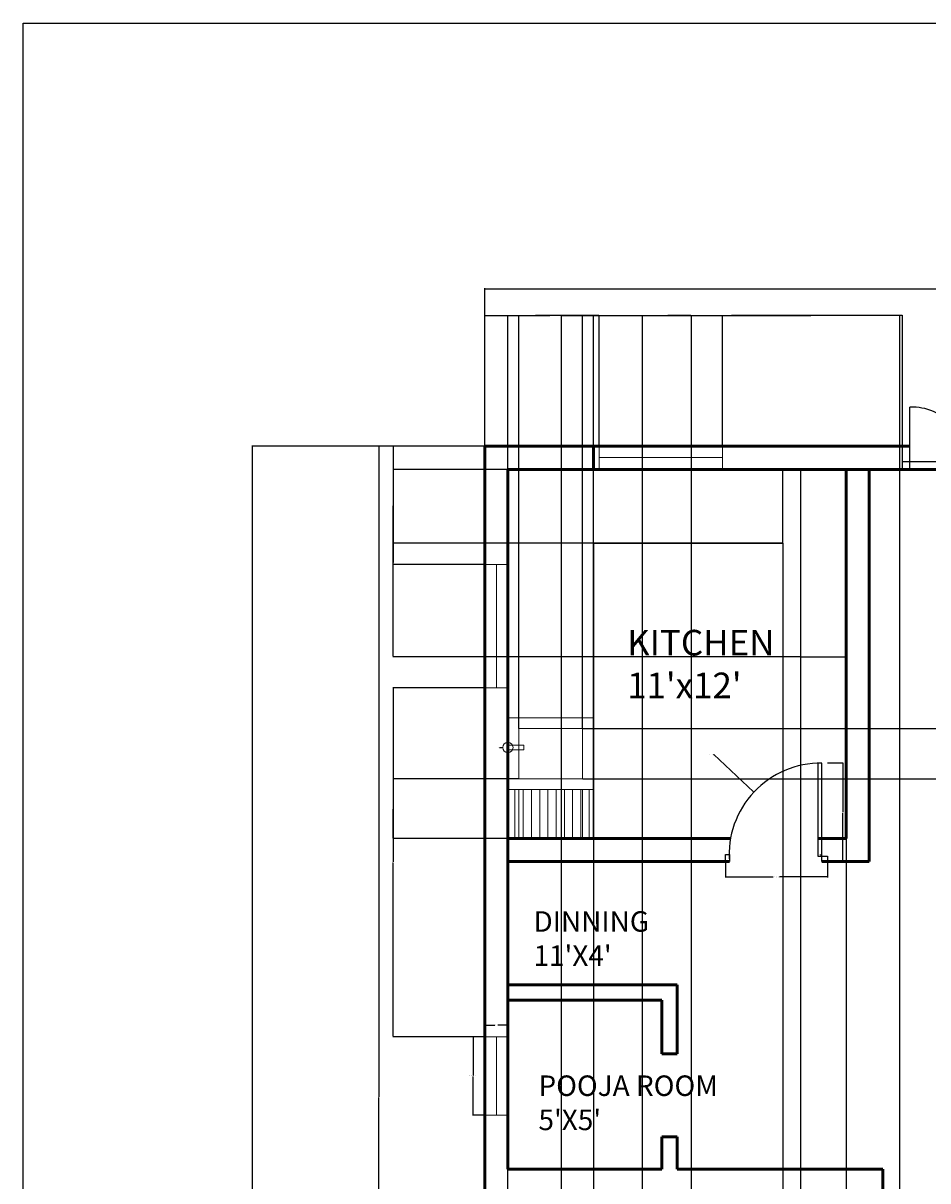
# Model space of a CAD drawing. Units: inches. Extents: x -177 to 2564, y -706 to 2548.
# Tile 3 of 4: x -177 to 176, y -266 to 186. Entities that reach past the tile are written whole.
import ezdxf

# ---------------------------------------------------------------- set-up
doc = ezdxf.new("R2010")
doc.units = ezdxf.units.IN
doc.header["$MEASUREMENT"] = 0
for name, color, linetype, lineweight in [('A-ANNO-DIMS', 2, 'Continuous', 18), ('A-ANNO-TTLB', 7, 'Continuous', 25), ('A-AREA-IDEN', 7, 'Continuous', 25), ('A-DOOR', 3, 'Continuous', 25), ('A-FLOR-CASE', 9, 'Continuous', 25), ('A-FLOR-FIXT', 8, 'Continuous', 18), ('A-GLAZ', 4, 'Continuous', 18), ('A-WALL', 7, 'Continuous', 50)]:
    doc.layers.add(name, color=color, linetype=linetype, lineweight=lineweight)
doc.styles.get("Standard").update_dxf_attribs({"font": 'arial.ttf'})
doc.dimstyles.get("Standard").update_dxf_attribs({"dimtxt": 0.18, "dimasz": 0.18, "dimexe": 0.18, "dimexo": 0.0625, "dimgap": 0.09, "dimtad": 0, "dimtih": 1, "dimtoh": 1, "dimdec": 0, "dimzin": 0, "dimdsep": 46, "dimlunit": 4, "dimtxsty": 'Standard', "dimcen": 0.09, "dimadec": 0, "dimazin": 0, "dimtfac": 1, "dimtdec": 0, "dimtofl": 0, "dimtmove": 0, "dimatfit": 3, "dimfxl": 1, "dimtolj": 1, "dimtzin": 0, "dimarcsym": 0})

# ---------------------------------------------------------------- blocks, each defined once
blk = doc.blocks.new('*D1')
at = {"layer": 'A-ANNO-DIMS', "color": 0, "lineweight": -2, "transparency": 16777216}
for p, q in [((3.47, 20.6), (3.47, 82.15)), ((3.65, 81.97), (192.07, 81.97)), ((381.29, 81.97), (192.87, 81.97)), ((381.47, 20.6), (381.47, 82.15))]:
    blk.add_line(p, q, dxfattribs=at)
at = {"layer": 'A-ANNO-DIMS', "color": 0, "transparency": 16777216}
for points in [[(3.65, 82), (3.65, 81.94), (3.47, 81.97)], [(381.29, 82), (381.29, 81.94), (381.47, 81.97)]]:
    blk.add_solid(points, dxfattribs=at)
at = {"layer": 'Defpoints', "color": 0, "transparency": 16777216}
for p in [(381.47, 81.97), (3.47, 20.54), (381.47, 20.54)]:
    blk.add_point(p, dxfattribs=at)
at = {"layer": 'A-ANNO-DIMS', "color": 0, "transparency": 16777216, "insert": (192.47, 81.97), "char_height": 0.18, "attachment_point": 5}
blk.add_mtext('\\A1;31\'-6"', dxfattribs=at)
blk = doc.blocks.new('*D2')
at = {"layer": 'A-ANNO-DIMS', "color": 0, "lineweight": -2, "transparency": 16777216}
for p, q in [((3.41, 20.54), (-38, 20.54)), ((-37.82, 20.36), (-37.82, -233.15)), ((-37.82, -487.01), (-37.82, -233.51)), ((3.41, -487.19), (-38, -487.19))]:
    blk.add_line(p, q, dxfattribs=at)
at = {"layer": 'A-ANNO-DIMS', "color": 0, "transparency": 16777216}
for points in [[(-37.85, 20.36), (-37.79, 20.36), (-37.82, 20.54)], [(-37.85, -487.01), (-37.79, -487.01), (-37.82, -487.19)]]:
    blk.add_solid(points, dxfattribs=at)
at = {"layer": 'Defpoints', "color": 0, "transparency": 16777216}
for p in [(3.47, 20.54), (-37.82, -487.19), (3.47, -487.19)]:
    blk.add_point(p, dxfattribs=at)
at = {"layer": 'A-ANNO-DIMS', "color": 0, "transparency": 16777216, "insert": (-37.82, -233.33), "char_height": 0.18, "attachment_point": 5}
blk.add_mtext('\\A1;42\'-4"', dxfattribs=at)
blk = doc.blocks.new('*D3')
at = {"layer": 'A-ANNO-DIMS', "color": 0, "lineweight": -2, "transparency": 16777216}
for p, q in [((3.41, 20.54), (-87.46, 20.54)), ((-87.28, 20.36), (-87.28, -294.78)), ((-87.28, -610.28), (-87.28, -295.15)), ((3.41, -610.46), (-87.46, -610.46))]:
    blk.add_line(p, q, dxfattribs=at)
at = {"layer": 'A-ANNO-DIMS', "color": 0, "transparency": 16777216}
for points in [[(-87.31, 20.36), (-87.25, 20.36), (-87.28, 20.54)], [(-87.31, -610.28), (-87.25, -610.28), (-87.28, -610.46)]]:
    blk.add_solid(points, dxfattribs=at)
at = {"layer": 'Defpoints', "color": 0, "transparency": 16777216}
for p in [(3.47, 20.54), (-87.28, -610.46), (3.47, -610.46)]:
    blk.add_point(p, dxfattribs=at)
at = {"layer": 'A-ANNO-DIMS', "color": 0, "transparency": 16777216, "insert": (-87.28, -294.96), "char_height": 0.18, "attachment_point": 5}
blk.add_mtext('\\A1;52\'-7"', dxfattribs=at)
blk = doc.blocks.new('WIN-48')
for p, q in [((0, 0), (9, 0)), ((9, 0), (4.59, 0)), ((4.59, 0), (4.59, -48.06)), ((9, -48.06), (0, -48.06))]:
    blk.add_line(p, q)
blk = doc.blocks.new('WIN-30')
for p, q in [((0, 30.54), (-9, 30.54)), ((-4.41, 0), (-4.41, 30.54)), ((0, 0), (-9, 0)), ((0, 0), (-4.41, 0))]:
    blk.add_line(p, q)
blk = doc.blocks.new('DOOR-SINGLE-36')
for p, q in [((1.57, 36.24), (0, 36.24)), ((0, 36.24), (0, 0)), ((1.57, -2.14), (1.57, 36.24)), ((1.57, 36.24), (1.57, 36.24)), ((-36.05, -2.14), (-36.05, 0.59)), ((-36.05, 0.59), (-34.54, 0.59)), ((-34.54, 0.59), (-34.54, -2.14)), ((0, 0), (3.72, 0)), ((3.72, 0), (3.72, -2.14)), ((3.72, -2.14), (1.57, -2.14))]:
    blk.add_line(p, q)
blk.add_arc((1.05, 0.56), 35.69, 89.1597, 184.3396)
blk = doc.blocks.new('DOOR-PAIR-44')
for p, q in [((0, 0), (0, 24.32)), ((44.01, 0), (44.01, 23.95)), ((-2.88, 0), (-2.88, 3.11)), ((-2.88, 3.11), (46.72, 3.11)), ((46.72, 0), (-2.88, 0)), ((-2.88, 0), (0, 0)), ((0, 0), (44.01, 0)), ((23.01, 0), (23.01, 3.55)), ((44.01, 0), (23.01, 0)), ((46.72, 0), (44.01, 0))]:
    blk.add_line(p, q)
for centre, radius, start, end in [((0.52, 1.77), 22.55, 355.4915, 91.326), ((45.7, 1.28), 22.73, 94.2755, 183.2347)]:
    blk.add_arc(centre, radius, start, end)
blk = doc.blocks.new('*D12')
at = {"layer": 'A-ANNO-DIMS', "color": 0, "lineweight": -2, "transparency": 16777216}
for p, q in [((3.41, -209.76), (-1.29, -209.76)), ((-1.11, -209.94), (-1.11, -224.85)), ((-1.11, -240.12), (-1.11, -225.22)), ((3.41, -240.3), (-1.29, -240.3))]:
    blk.add_line(p, q, dxfattribs=at)
at = {"layer": 'A-ANNO-DIMS', "color": 0, "transparency": 16777216}
for points in [[(-1.14, -209.94), (-1.08, -209.94), (-1.11, -209.76)], [(-1.14, -240.12), (-1.08, -240.12), (-1.11, -240.3)]]:
    blk.add_solid(points, dxfattribs=at)
at = {"layer": 'Defpoints', "color": 0, "transparency": 16777216}
for p in [(-1.11, -209.76), (3.47, -209.76), (3.47, -240.3)]:
    blk.add_point(p, dxfattribs=at)
at = {"layer": 'A-ANNO-DIMS', "color": 0, "transparency": 16777216, "insert": (-1.11, -225.03), "char_height": 0.18, "attachment_point": 5}
blk.add_mtext('\\A1;WINDOW W2 2\'-6 1/2" TYP.', dxfattribs=at)
blk = doc.blocks.new('*D13')
at = {"layer": 'A-ANNO-DIMS', "color": 0, "lineweight": -2, "transparency": 16777216}
for p, q in [((3.47, -209.7), (3.47, -205)), ((3.65, -205.18), (7.33, -205.18)), ((12.29, -205.18), (8.61, -205.18)), ((12.47, -209.7), (12.47, -205))]:
    blk.add_line(p, q, dxfattribs=at)
at = {"layer": 'A-ANNO-DIMS', "color": 0, "transparency": 16777216}
for points in [[(3.65, -205.15), (3.65, -205.21), (3.47, -205.18)], [(12.29, -205.15), (12.29, -205.21), (12.47, -205.18)]]:
    blk.add_solid(points, dxfattribs=at)
at = {"layer": 'Defpoints', "color": 0, "transparency": 16777216}
for p in [(12.47, -205.18), (3.47, -209.76), (12.47, -209.76)]:
    blk.add_point(p, dxfattribs=at)
at = {"layer": 'A-ANNO-DIMS', "color": 0, "transparency": 16777216, "insert": (7.97, -205.18), "char_height": 0.18, "attachment_point": 5}
blk.add_mtext('\\A1;0\'-9" TYP.', dxfattribs=at)
blk = doc.blocks.new('*D16')
at = {"layer": 'A-ANNO-DIMS', "color": 0, "lineweight": -2, "transparency": 16777216}
for p, q in [((97.36, -141.53), (97.36, -147.61)), ((137.13, -141.53), (137.13, -147.61)), ((97.54, -147.43), (116, -147.43)), ((136.95, -147.43), (118.49, -147.43))]:
    blk.add_line(p, q, dxfattribs=at)
at = {"layer": 'A-ANNO-DIMS', "color": 0, "transparency": 16777216}
for points in [[(97.54, -147.4), (97.54, -147.46), (97.36, -147.43)], [(136.95, -147.4), (136.95, -147.46), (137.13, -147.43)]]:
    blk.add_solid(points, dxfattribs=at)
at = {"layer": 'Defpoints', "color": 0, "transparency": 16777216}
for p in [(97.36, -141.46), (137.13, -141.46), (137.13, -147.43)]:
    blk.add_point(p, dxfattribs=at)
at = {"layer": 'A-ANNO-DIMS', "color": 0, "transparency": 16777216, "insert": (117.24, -147.43), "char_height": 0.18, "attachment_point": 5}
blk.add_mtext('\\A1;DOOR D1 3\'-4" TYP.', dxfattribs=at)
blk = doc.blocks.new('*D17')
at = {"layer": 'A-ANNO-DIMS', "color": 0, "lineweight": -2, "transparency": 16777216}
for p, q in [((137.19, -102.94), (143.28, -102.94)), ((143.1, -103.12), (143.1, -122.02)), ((143.1, -141.28), (143.1, -122.38)), ((137.19, -141.46), (143.28, -141.46))]:
    blk.add_line(p, q, dxfattribs=at)
at = {"layer": 'A-ANNO-DIMS', "color": 0, "transparency": 16777216}
for points in [[(143.07, -103.12), (143.13, -103.12), (143.1, -102.94)], [(143.07, -141.28), (143.13, -141.28), (143.1, -141.46)]]:
    blk.add_solid(points, dxfattribs=at)
at = {"layer": 'Defpoints', "color": 0, "transparency": 16777216}
for p in [(137.13, -102.94), (143.1, -102.94), (137.13, -141.46)]:
    blk.add_point(p, dxfattribs=at)
at = {"layer": 'A-ANNO-DIMS', "color": 0, "transparency": 16777216, "insert": (143.1, -122.2), "char_height": 0.18, "attachment_point": 5}
blk.add_mtext('\\A1;3\'-2 1/2" TYP.', dxfattribs=at)
blk = doc.blocks.new('*D22')
at = {"layer": 'A-ANNO-DIMS', "color": 0, "lineweight": -2, "transparency": 16777216}
for p, q in [((33.37, -291.35), (33.37, 71.74)), ((33.55, 71.56), (98.96, 71.56)), ((165.15, 71.56), (99.74, 71.56)), ((165.33, -291.35), (165.33, 71.74))]:
    blk.add_line(p, q, dxfattribs=at)
at = {"layer": 'A-ANNO-DIMS', "color": 0, "transparency": 16777216}
for points in [[(33.55, 71.59), (33.55, 71.53), (33.37, 71.56)], [(165.15, 71.59), (165.15, 71.53), (165.33, 71.56)]]:
    blk.add_solid(points, dxfattribs=at)
at = {"layer": 'Defpoints', "color": 0, "transparency": 16777216}
for p in [(165.33, 71.56), (33.37, -291.42), (165.33, -291.42)]:
    blk.add_point(p, dxfattribs=at)
at = {"layer": 'A-ANNO-DIMS', "color": 0, "transparency": 16777216, "insert": (99.35, 71.56), "char_height": 0.18, "attachment_point": 5}
blk.add_mtext('\\A1;11\'-0"', dxfattribs=at)
blk = doc.blocks.new('*D26')
at = {"layer": 'A-ANNO-DIMS', "color": 0, "lineweight": -2, "transparency": 16777216}
for p, q in [((64.94, -324.62), (64.94, 71.74)), ((65.12, 71.56), (74.18, 71.56)), ((83.88, 71.56), (74.82, 71.56)), ((84.06, -343.44), (84.06, 71.74))]:
    blk.add_line(p, q, dxfattribs=at)
at = {"layer": 'A-ANNO-DIMS', "color": 0, "transparency": 16777216}
for points in [[(65.12, 71.59), (65.12, 71.53), (64.94, 71.56)], [(83.88, 71.59), (83.88, 71.53), (84.06, 71.56)]]:
    blk.add_solid(points, dxfattribs=at)
at = {"layer": 'Defpoints', "color": 0, "transparency": 16777216}
for p in [(84.06, 71.56), (64.94, -324.69), (84.06, -343.5)]:
    blk.add_point(p, dxfattribs=at)
at = {"layer": 'A-ANNO-DIMS', "color": 0, "transparency": 16777216, "insert": (74.5, 71.56), "char_height": 0.18, "attachment_point": 5}
blk.add_mtext('\\A1;1\'-7"', dxfattribs=at)
blk = doc.blocks.new('*D28')
at = {"layer": 'A-ANNO-DIMS', "color": 0, "lineweight": -2, "transparency": 16777216}
for p, q in [((12.47, -270.4), (12.47, 71.74)), ((12.65, 71.56), (22.6, 71.56)), ((33.19, 71.56), (23.24, 71.56)), ((33.37, -291.35), (33.37, 71.74))]:
    blk.add_line(p, q, dxfattribs=at)
at = {"layer": 'A-ANNO-DIMS', "color": 0, "transparency": 16777216}
for points in [[(12.65, 71.59), (12.65, 71.53), (12.47, 71.56)], [(33.19, 71.59), (33.19, 71.53), (33.37, 71.56)]]:
    blk.add_solid(points, dxfattribs=at)
at = {"layer": 'Defpoints', "color": 0, "transparency": 16777216}
for p in [(33.37, 71.56), (12.47, -270.46), (33.37, -291.42)]:
    blk.add_point(p, dxfattribs=at)
at = {"layer": 'A-ANNO-DIMS', "color": 0, "transparency": 16777216, "insert": (22.92, 71.56), "char_height": 0.18, "attachment_point": 5}
blk.add_mtext('\\A1;1\'-9"', dxfattribs=at)
blk = doc.blocks.new('*D30')
at = {"layer": 'A-ANNO-DIMS', "color": 0, "lineweight": -2, "transparency": 16777216}
for p, q in [((12.47, -85.26), (12.47, 71.74)), ((12.65, 71.56), (28.65, 71.56)), ((45.73, 71.56), (29.73, 71.56)), ((45.91, -85.26), (45.91, 71.74))]:
    blk.add_line(p, q, dxfattribs=at)
at = {"layer": 'A-ANNO-DIMS', "color": 0, "transparency": 16777216}
for points in [[(12.65, 71.59), (12.65, 71.53), (12.47, 71.56)], [(45.73, 71.59), (45.73, 71.53), (45.91, 71.56)]]:
    blk.add_solid(points, dxfattribs=at)
at = {"layer": 'Defpoints', "color": 0, "transparency": 16777216}
for p in [(45.91, 71.56), (12.47, -85.33), (45.91, -85.33)]:
    blk.add_point(p, dxfattribs=at)
at = {"layer": 'A-ANNO-DIMS', "color": 0, "transparency": 16777216, "insert": (29.19, 71.56), "char_height": 0.18, "attachment_point": 5}
blk.add_mtext('\\A1;2\'-9 1/2"', dxfattribs=at)
blk = doc.blocks.new('*D31')
at = {"layer": 'A-ANNO-DIMS', "color": 0, "lineweight": -2, "transparency": 16777216}
for p, q in [((119.69, 11.54), (-32.41, 11.54)), ((-32.23, 11.36), (-32.23, -2.66)), ((-32.23, -17.03), (-32.23, -3.02)), ((119.69, -17.21), (-32.41, -17.21))]:
    blk.add_line(p, q, dxfattribs=at)
at = {"layer": 'A-ANNO-DIMS', "color": 0, "transparency": 16777216}
for points in [[(-32.26, 11.36), (-32.2, 11.36), (-32.23, 11.54)], [(-32.26, -17.03), (-32.2, -17.03), (-32.23, -17.21)]]:
    blk.add_solid(points, dxfattribs=at)
at = {"layer": 'Defpoints', "color": 0, "transparency": 16777216}
for p in [(119.76, 11.54), (-32.23, -17.21), (119.76, -17.21)]:
    blk.add_point(p, dxfattribs=at)
at = {"layer": 'A-ANNO-DIMS', "color": 0, "transparency": 16777216, "insert": (-32.23, -2.84), "char_height": 0.18, "attachment_point": 5}
blk.add_mtext('\\A1;2\'-4 1/2"', dxfattribs=at)
blk = doc.blocks.new('*D32')
at = {"layer": 'A-ANNO-DIMS', "color": 0, "lineweight": -2, "transparency": 16777216}
for p, q in [((45.91, -17.28), (45.91, -646.34)), ((119.76, -17.28), (119.76, -646.34)), ((46.09, -646.16), (82.5, -646.16)), ((119.58, -646.16), (83.16, -646.16))]:
    blk.add_line(p, q, dxfattribs=at)
at = {"layer": 'A-ANNO-DIMS', "color": 0, "transparency": 16777216}
for points in [[(46.09, -646.13), (46.09, -646.19), (45.91, -646.16)], [(119.58, -646.13), (119.58, -646.19), (119.76, -646.16)]]:
    blk.add_solid(points, dxfattribs=at)
at = {"layer": 'Defpoints', "color": 0, "transparency": 16777216}
for p in [(45.91, -17.21), (119.76, -17.21), (119.76, -646.16)]:
    blk.add_point(p, dxfattribs=at)
at = {"layer": 'A-ANNO-DIMS', "color": 0, "transparency": 16777216, "insert": (82.83, -646.16), "char_height": 0.18, "attachment_point": 5}
blk.add_mtext('\\A1;6\'-2"', dxfattribs=at)
blk = doc.blocks.new('*D33')
at = {"layer": 'A-ANNO-DIMS', "color": 0, "lineweight": -2, "transparency": 16777216}
for p, q in [((126.64, -61.62), (126.64, -646.34)), ((144.47, -61.62), (144.47, -646.34)), ((126.82, -646.16), (135.24, -646.16)), ((144.29, -646.16), (135.88, -646.16))]:
    blk.add_line(p, q, dxfattribs=at)
at = {"layer": 'A-ANNO-DIMS', "color": 0, "transparency": 16777216}
for points in [[(126.82, -646.13), (126.82, -646.19), (126.64, -646.16)], [(144.29, -646.13), (144.29, -646.19), (144.47, -646.16)]]:
    blk.add_solid(points, dxfattribs=at)
at = {"layer": 'Defpoints', "color": 0, "transparency": 16777216}
for p in [(126.64, -61.56), (144.47, -61.56), (144.47, -646.16)]:
    blk.add_point(p, dxfattribs=at)
at = {"layer": 'A-ANNO-DIMS', "color": 0, "transparency": 16777216, "insert": (135.56, -646.16), "char_height": 0.18, "attachment_point": 5}
blk.add_mtext('\\A1;1\'-6"', dxfattribs=at)
blk = doc.blocks.new('*D34')
at = {"layer": 'A-ANNO-DIMS', "color": 0, "lineweight": -2, "transparency": 16777216}
for p, q in [((126.58, 11.54), (-32.41, 11.54)), ((-32.23, 11.36), (-32.23, -24.83)), ((-32.23, -61.38), (-32.23, -25.19)), ((126.58, -61.56), (-32.41, -61.56))]:
    blk.add_line(p, q, dxfattribs=at)
at = {"layer": 'A-ANNO-DIMS', "color": 0, "transparency": 16777216}
for points in [[(-32.26, 11.36), (-32.2, 11.36), (-32.23, 11.54)], [(-32.26, -61.38), (-32.2, -61.38), (-32.23, -61.56)]]:
    blk.add_solid(points, dxfattribs=at)
at = {"layer": 'Defpoints', "color": 0, "transparency": 16777216}
for p in [(-32.23, 11.54), (126.64, 11.54), (126.64, -61.56)]:
    blk.add_point(p, dxfattribs=at)
at = {"layer": 'A-ANNO-DIMS', "color": 0, "transparency": 16777216, "insert": (-32.23, -25.01), "char_height": 0.18, "attachment_point": 5}
blk.add_mtext('\\A1;6\'-1"', dxfattribs=at)
blk = doc.blocks.new('*D35')
at = {"layer": 'A-ANNO-DIMS', "color": 0, "lineweight": -2, "transparency": 16777216}
for p, q in [((16.73, -89.52), (16.73, 71.74)), ((16.91, 71.56), (28.86, 71.56)), ((41.47, 71.56), (29.52, 71.56)), ((41.65, -89.52), (41.65, 71.74))]:
    blk.add_line(p, q, dxfattribs=at)
at = {"layer": 'A-ANNO-DIMS', "color": 0, "transparency": 16777216}
for points in [[(16.91, 71.59), (16.91, 71.53), (16.73, 71.56)], [(41.47, 71.59), (41.47, 71.53), (41.65, 71.56)]]:
    blk.add_solid(points, dxfattribs=at)
at = {"layer": 'Defpoints', "color": 0, "transparency": 16777216}
for p in [(41.65, 71.56), (16.73, -89.59), (41.65, -89.59)]:
    blk.add_point(p, dxfattribs=at)
at = {"layer": 'A-ANNO-DIMS', "color": 0, "transparency": 16777216, "insert": (29.19, 71.56), "char_height": 0.18, "attachment_point": 5}
blk.add_mtext('\\A1;2\'-1"', dxfattribs=at)
blk = doc.blocks.new('*D36')
at = {"layer": 'A-ANNO-DIMS', "color": 0, "lineweight": -2, "transparency": 16777216}
for p, q in [((41.71, -89.59), (417.35, -89.59)), ((417.17, -89.77), (417.17, -99.17)), ((417.17, -108.95), (417.17, -99.54)), ((41.71, -109.13), (417.35, -109.13))]:
    blk.add_line(p, q, dxfattribs=at)
at = {"layer": 'A-ANNO-DIMS', "color": 0, "transparency": 16777216}
for points in [[(417.14, -89.77), (417.2, -89.77), (417.17, -89.59)], [(417.14, -108.95), (417.2, -108.95), (417.17, -109.13)]]:
    blk.add_solid(points, dxfattribs=at)
at = {"layer": 'Defpoints', "color": 0, "transparency": 16777216}
for p in [(41.65, -89.59), (41.65, -109.13), (417.17, -109.13)]:
    blk.add_point(p, dxfattribs=at)
at = {"layer": 'A-ANNO-DIMS', "color": 0, "transparency": 16777216, "insert": (417.17, -99.36), "char_height": 0.18, "attachment_point": 5}
blk.add_mtext('\\A1;1\'-7 1/2"', dxfattribs=at)
blk = doc.blocks.new('*D37')
at = {"layer": 'A-ANNO-DIMS', "color": 0, "lineweight": -2, "transparency": 16777216}
for p, q in [((16.67, -109.13), (-32.41, -109.13)), ((-32.23, -109.31), (-32.23, -120.61)), ((-32.23, -132.28), (-32.23, -120.98)), ((12.41, -132.46), (-32.41, -132.46))]:
    blk.add_line(p, q, dxfattribs=at)
at = {"layer": 'A-ANNO-DIMS', "color": 0, "transparency": 16777216}
for points in [[(-32.26, -109.31), (-32.2, -109.31), (-32.23, -109.13)], [(-32.26, -132.28), (-32.2, -132.28), (-32.23, -132.46)]]:
    blk.add_solid(points, dxfattribs=at)
at = {"layer": 'Defpoints', "color": 0, "transparency": 16777216}
for p in [(-32.23, -109.13), (16.73, -109.13), (12.47, -132.46)]:
    blk.add_point(p, dxfattribs=at)
at = {"layer": 'A-ANNO-DIMS', "color": 0, "transparency": 16777216, "insert": (-32.23, -120.8), "char_height": 0.18, "attachment_point": 5}
blk.add_mtext('\\A1;1\'-11 1/2"', dxfattribs=at)
blk = doc.blocks.new('*D50')
at = {"layer": 'A-ANNO-DIMS', "color": 0, "lineweight": -2, "transparency": 16777216}
for p, q in [((3.47, 20.6), (3.47, 71.74)), ((3.65, 71.56), (25.24, 71.56)), ((47.91, 71.56), (26.32, 71.56)), ((48.09, 20.6), (48.09, 71.74))]:
    blk.add_line(p, q, dxfattribs=at)
at = {"layer": 'A-ANNO-DIMS', "color": 0, "transparency": 16777216}
for points in [[(3.65, 71.59), (3.65, 71.53), (3.47, 71.56)], [(47.91, 71.59), (47.91, 71.53), (48.09, 71.56)]]:
    blk.add_solid(points, dxfattribs=at)
at = {"layer": 'Defpoints', "color": 0, "transparency": 16777216}
for p in [(48.09, 71.56), (3.47, 20.54), (48.09, 20.54)]:
    blk.add_point(p, dxfattribs=at)
at = {"layer": 'A-ANNO-DIMS', "color": 0, "transparency": 16777216, "insert": (25.78, 71.56), "char_height": 0.18, "attachment_point": 5}
blk.add_mtext('\\A1;3\'-8 1/2"', dxfattribs=at)
blk = doc.blocks.new('*D51')
at = {"layer": 'A-ANNO-DIMS', "color": 0, "lineweight": -2, "transparency": 16777216}
for p, q in [((96.15, 20.6), (96.15, 71.74)), ((96.33, 71.56), (130.67, 71.56)), ((166.23, 71.56), (131.89, 71.56)), ((166.41, 20.6), (166.41, 71.74))]:
    blk.add_line(p, q, dxfattribs=at)
at = {"layer": 'A-ANNO-DIMS', "color": 0, "transparency": 16777216}
for points in [[(96.33, 71.59), (96.33, 71.53), (96.15, 71.56)], [(166.23, 71.59), (166.23, 71.53), (166.41, 71.56)]]:
    blk.add_solid(points, dxfattribs=at)
at = {"layer": 'Defpoints', "color": 0, "transparency": 16777216}
for p in [(166.41, 71.56), (96.15, 20.54), (166.41, 20.54)]:
    blk.add_point(p, dxfattribs=at)
at = {"layer": 'A-ANNO-DIMS', "color": 0, "transparency": 16777216, "insert": (131.28, 71.56), "char_height": 0.18, "attachment_point": 5}
blk.add_mtext('\\A1;5\'-10 1/2"', dxfattribs=at)
blk = doc.blocks.new('*D53')
at = {"layer": 'A-ANNO-DIMS', "color": 0, "lineweight": -2, "transparency": 16777216}
for p, q in [((3.41, 20.54), (-32.41, 20.54)), ((-32.23, 20.36), (-32.23, -2.36)), ((-32.23, -25.45), (-32.23, -2.73)), ((3.41, -25.63), (-32.41, -25.63))]:
    blk.add_line(p, q, dxfattribs=at)
at = {"layer": 'A-ANNO-DIMS', "color": 0, "transparency": 16777216}
for points in [[(-32.26, 20.36), (-32.2, 20.36), (-32.23, 20.54)], [(-32.26, -25.45), (-32.2, -25.45), (-32.23, -25.63)]]:
    blk.add_solid(points, dxfattribs=at)
at = {"layer": 'Defpoints', "color": 0, "transparency": 16777216}
for p in [(-32.23, 20.54), (3.47, 20.54), (3.47, -25.63)]:
    blk.add_point(p, dxfattribs=at)
at = {"layer": 'A-ANNO-DIMS', "color": 0, "transparency": 16777216, "insert": (-32.23, -2.55), "char_height": 0.18, "attachment_point": 5}
blk.add_mtext('\\A1;3\'-10"', dxfattribs=at)
blk = doc.blocks.new('*D55')
at = {"layer": 'A-ANNO-DIMS', "color": 0, "lineweight": -2, "transparency": 16777216}
for p, q in [((3.41, -73.69), (-32.41, -73.69)), ((-32.23, -73.87), (-32.23, -141.54)), ((-32.23, -209.58), (-32.23, -141.9)), ((3.41, -209.76), (-32.41, -209.76))]:
    blk.add_line(p, q, dxfattribs=at)
at = {"layer": 'A-ANNO-DIMS', "color": 0, "transparency": 16777216}
for points in [[(-32.26, -73.87), (-32.2, -73.87), (-32.23, -73.69)], [(-32.26, -209.58), (-32.2, -209.58), (-32.23, -209.76)]]:
    blk.add_solid(points, dxfattribs=at)
at = {"layer": 'Defpoints', "color": 0, "transparency": 16777216}
for p in [(3.47, -73.69), (-32.23, -209.76), (3.47, -209.76)]:
    blk.add_point(p, dxfattribs=at)
at = {"layer": 'A-ANNO-DIMS', "color": 0, "transparency": 16777216, "insert": (-32.23, -141.72), "char_height": 0.18, "attachment_point": 5}
blk.add_mtext('\\A1;11\'-4"', dxfattribs=at)
blk = doc.blocks.new('*D62')
at = {"layer": 'A-ANNO-DIMS', "color": 0, "lineweight": -2, "transparency": 16777216}
for p, q in [((9.26, -96.93), (10.28, -96.94)), ((12.38, -96.96), (12.56, -96.96)), ((12.47, -97.05), (12.47, -96.87))]:
    blk.add_line(p, q, dxfattribs=at)
at = {"layer": 'A-ANNO-DIMS', "color": 0, "transparency": 16777216}
blk.add_solid([(10.28, -96.91), (10.28, -96.97), (10.46, -96.94)], dxfattribs=at)
at = {"layer": 'Defpoints', "color": 0, "transparency": 16777216}
for p in [(10.46, -96.94), (14.48, -96.98)]:
    blk.add_point(p, dxfattribs=at)
at = {"layer": 'A-ANNO-DIMS', "color": 0, "transparency": 16777216, "insert": (8.83, -96.93), "char_height": 0.18, "attachment_point": 5}
blk.add_mtext('\\A1;∅0\'-4"', dxfattribs=at)
blk = doc.blocks.new('*D63')
at = {"layer": 'A-ANNO-DIMS', "color": 0, "lineweight": -2, "transparency": 16777216}
for p, q in [((92.69, -99.64), (92.87, -99.64)), ((92.87, -99.64), (108.33, -114.19)), ((134.37, -138.76), (134.55, -138.76)), ((134.46, -138.85), (134.46, -138.67))]:
    blk.add_line(p, q, dxfattribs=at)
at = {"layer": 'A-ANNO-DIMS', "color": 0, "transparency": 16777216}
blk.add_solid([(108.36, -114.17), (108.31, -114.21), (108.47, -114.31)], dxfattribs=at)
at = {"layer": 'Defpoints', "color": 0, "transparency": 16777216}
for p in [(108.47, -114.31), (134.46, -138.76)]:
    blk.add_point(p, dxfattribs=at)
at = {"layer": 'A-ANNO-DIMS', "color": 0, "transparency": 16777216, "insert": (91.8, -99.64), "char_height": 0.18, "attachment_point": 5}
blk.add_mtext('\\A1;6X R2\'-11 1/2"', dxfattribs=at)

msp = doc.modelspace()

# ---------------------------------------------------------------- linework, layer by layer
at = {"layer": 'A-ANNO-TTLB'}
msp.add_lwpolyline([(-176.6, 185.58), (523.32, 185.58), (523.32, -705.52), (-176.6, -705.52)], close=True, dxfattribs=at)
at = {"layer": 'A-DOOR'}
for p, q in [((166.41, 11.54), (166.41, 20.54)), ((97.36, -141.46), (98.87, -141.46))]:
    msp.add_line(p, q, dxfattribs=at)
at = {"layer": 'A-FLOR-CASE'}
for p, q in [((119.76, -17.21), (119.76, 11.54)), ((119.76, 11.54), (126.64, 11.54)), ((126.64, 11.54), (126.64, -61.56)), ((45.91, -132.46), (45.91, -17.21)), ((45.91, -17.21), (119.76, -17.21)), ((126.64, -61.56), (144.47, -61.56)), ((12.47, -132.46), (45.91, -132.46))]:
    msp.add_line(p, q, dxfattribs=at)
msp.add_lwpolyline([(45.91, -17.21), (45.91, -132.46), (12.47, -132.46), (12.47, 11.54)], dxfattribs=at)
at = {"layer": 'A-FLOR-FIXT'}
for p, q in [((45.91, -85.33), (12.47, -85.33)), ((12.47, -85.33), (12.47, -98.97)), ((12.47, -85.33), (12.47, -96.02)), ((45.91, -132.46), (45.91, -85.33)), ((41.65, -89.59), (16.73, -89.59)), ((16.73, -89.59), (16.73, -109.13)), ((41.65, -109.13), (41.65, -89.59)), ((12.47, -96.02), (18.74, -96.02)), ((18.74, -97.91), (12.47, -97.91)), ((18.74, -96.02), (18.74, -97.91)), ((16.73, -109.13), (41.65, -109.13)), ((12.47, -132.46), (12.47, -113.39)), ((12.47, -113.39), (45.91, -113.39)), ((12.47, -113.39), (15.24, -113.39)), ((12.47, -113.39), (12.47, -132.46)), ((15.24, -113.39), (15.24, -132.46)), ((16.73, -113.39), (16.73, -132.46)), ((18.46, -113.39), (18.46, -132.46)), ((21.67, -113.39), (21.67, -132.46)), ((24.88, -113.39), (24.88, -132.46)), ((28.09, -113.39), (28.09, -132.46)), ((31.31, -113.39), (31.31, -132.46)), ((34.52, -113.39), (34.52, -132.46)), ((37.73, -113.39), (37.73, -132.46)), ((40.95, -113.39), (40.95, -132.46)), ((41.65, -132.46), (41.65, -113.39)), ((44.16, -113.39), (44.16, -132.46)), ((12.47, -132.46), (45.91, -132.46))]:
    msp.add_line(p, q, dxfattribs=at)
msp.add_circle((12.47, -96.96), 2.01, dxfattribs=at)
at = {"layer": 'A-GLAZ'}
for p, q in [((3.47, -73.69), (12.47, -73.69)), ((3.47, -209.76), (3.47, -240.3))]:
    msp.add_line(p, q, dxfattribs=at)
at = {"layer": 'A-WALL'}
for p, q in [((3.47, -483.46), (3.47, 20.54)), ((3.47, 20.54), (12.47, 20.54)), ((12.47, 20.54), (169.3, 20.54)), ((12.47, 11.54), (372.47, 11.54)), ((12.47, 11.54), (12.47, -261.46)), ((12.47, 11.54), (144.47, 11.54)), ((144.47, 11.54), (144.47, -132.46)), ((153.47, -141.46), (153.47, 11.54)), ((12.47, -132.46), (12.47, -141.46)), ((99.33, -132.46), (12.47, -132.46)), ((144.47, -132.46), (133.41, -132.46)), ((12.47, -141.46), (98.87, -141.46)), ((12.47, -141.46), (12.47, -189.46)), ((134.98, -141.46), (144.47, -141.46)), ((144.47, -141.46), (153.47, -141.46)), ((144.47, -141.46), (153.47, -141.46)), ((12.47, -189.46), (72.47, -189.46)), ((72.47, -189.46), (78.47, -189.46)), ((78.47, -189.46), (78.47, -216.41)), ((72.47, -195.46), (12.47, -195.46)), ((12.47, -195.46), (12.47, -255.46)), ((12.47, -195.46), (12.47, -209.76)), ((72.47, -216.41), (72.47, -195.46)), ((78.47, -216.41), (72.47, -216.41)), ((72.47, -255.46), (72.47, -248.84)), ((72.47, -248.84), (78.5, -248.84)), ((78.5, -248.84), (78.5, -261.46)), ((72.47, -255.46), (72.47, -261.46)), ((72.47, -261.46), (12.47, -261.46)), ((12.47, -261.46), (72.47, -261.46)), ((78.5, -261.46), (158.78, -261.46)), ((158.78, -261.46), (158.78, -270.46))]:
    msp.add_line(p, q, dxfattribs=at)
msp.add_lwpolyline([(12.47, 20.54), (45.91, 20.54), (45.91, 11.54)], dxfattribs=at)

# ---------------------------------------------------------------- block references
at = {"layer": 'A-DOOR'}
for name, p in [('DOOR-PAIR-44', (169.3, 11.54)), ('DOOR-SINGLE-36', (133.41, -139.32))]:
    msp.add_blockref(name, p, dxfattribs=at)
at = {"layer": 'A-GLAZ', "rotation": 89.99999999999987}
msp.add_blockref('WIN-48', (48.09, 11.54), dxfattribs=at)
at = {"layer": 'A-GLAZ'}
for name, p in [('WIN-48', (3.47, -25.63)), ('WIN-30', (12.47, -240.3))]:
    msp.add_blockref(name, p, dxfattribs=at)

# ---------------------------------------------------------------- texts
at = {"layer": 'A-AREA-IDEN', "attachment_point": 1}
for s, width, insert, char_height in [("KITCHEN \\P11'x12'", 38.4012, (58.98, -51.06), 10), ("DINNING\\P11'X4'", 0.2169, (22.47, -160.8), 8)]:
    msp.add_mtext_dynamic_manual_height_columns(s, width=width, gutter_width=1, heights=[0], dxfattribs=dict(at, insert=insert, char_height=char_height))
at = {"layer": 'A-AREA-IDEN', "insert": (24.41, -224.86), "char_height": 8, "attachment_point": 1}
msp.add_mtext("POOJA ROOM\\P5'X5'", dxfattribs=at)

# ---------------------------------------------------------------- dimensions: what is measured, and where the dimension line sits
at = {"layer": 'A-ANNO-DIMS'}
for base, p1, p2, override, picture, middle in [((381.47, 81.97), (3.47, 20.54), (381.47, 20.54), {"dimclrd": 0, "dimclre": 0, "dimclrt": 0}, '*D1', (192.47, 81.97)), ((48.09, 71.56), (3.47, 20.54), (48.09, 20.54), {"dimdec": 1, "dimlfac": 1, "dimrnd": 0, "dimzin": 1, "dimdsep": 46, "dimlunit": 4, "dimfrac": 2}, '*D50', (25.78, 71.56)), ((45.91, 71.56), (12.47, -85.33), (45.91, -85.33), {"dimdec": 1, "dimlfac": 1, "dimrnd": 0, "dimzin": 1, "dimdsep": 46, "dimlunit": 4, "dimfrac": 2}, '*D30', (29.19, 71.56)), ((33.37, 71.56), (12.47, -270.46), (33.37, -291.42), {"dimdec": 1, "dimlfac": 1, "dimrnd": 0, "dimzin": 1, "dimdsep": 46, "dimlunit": 4, "dimfrac": 2}, '*D28', (22.92, 71.56)), ((41.65, 71.56), (16.73, -89.59), (41.65, -89.59), {"dimdec": 1, "dimlfac": 1, "dimrnd": 0, "dimzin": 1, "dimdsep": 46, "dimlunit": 4, "dimfrac": 2}, '*D35', (29.19, 71.56)), ((165.33, 71.56), (33.37, -291.42), (165.33, -291.42), {"dimdec": 1, "dimlfac": 1, "dimrnd": 0, "dimzin": 1, "dimdsep": 46, "dimlunit": 4, "dimfrac": 2}, '*D22', (99.35, 71.56)), ((84.06, 71.56), (64.94, -324.69), (84.06, -343.5), {"dimdec": 1, "dimlfac": 1, "dimrnd": 0, "dimzin": 1, "dimdsep": 46, "dimlunit": 4, "dimfrac": 2}, '*D26', (74.5, 71.56)), ((166.41, 71.56), (96.15, 20.54), (166.41, 20.54), {"dimdec": 1, "dimlfac": 1, "dimrnd": 0, "dimzin": 1, "dimdsep": 46, "dimlunit": 4, "dimfrac": 2}, '*D51', (131.28, 71.56)), ((119.7563, -646.1645), (45.9113, -17.2143), (119.7563, -17.2143), {"dimdec": 1, "dimlfac": 1, "dimrnd": 0, "dimzin": 1, "dimdsep": 46, "dimlunit": 4, "dimfrac": 2}, '*D32', (82.8338, -646.1645)), ((144.47, -646.16), (126.64, -61.56), (144.47, -61.56), {"dimdec": 1, "dimlfac": 1, "dimrnd": 0, "dimzin": 1, "dimdsep": 46, "dimlunit": 4, "dimfrac": 2}, '*D33', (135.56, -646.16))]:
    dim = msp.add_linear_dim(base=base, p1=p1, p2=p2, dimstyle='Standard', override=override, dxfattribs=at)
    dim.commit()
    dim.dimension.update_dxf_attribs({"geometry": picture, "text_midpoint": middle})
for base, p1, p2, override, picture, middle in [((-87.28, -610.46), (3.47, 20.54), (3.47, -610.46), {"dimclrd": 0, "dimclre": 0, "dimclrt": 0}, '*D3', (-87.28, -294.96)), ((-37.82, -487.19), (3.47, 20.54), (3.47, -487.19), {"dimclrd": 0, "dimclre": 0, "dimclrt": 0}, '*D2', (-37.82, -233.33)), ((-32.23, 20.54), (3.47, -25.63), (3.47, 20.54), {"dimdec": 1, "dimlfac": 1, "dimrnd": 0, "dimzin": 1, "dimdsep": 46, "dimlunit": 4, "dimfrac": 2}, '*D53', (-32.23, -2.55)), ((-32.2267, -17.2143), (119.7563, 11.5355), (119.7563, -17.2143), {"dimdec": 1, "dimlfac": 1, "dimrnd": 0, "dimzin": 1, "dimdsep": 46, "dimlunit": 4, "dimfrac": 2}, '*D31', (-32.2267, -2.8394)), ((-32.23, 11.54), (126.64, -61.56), (126.64, 11.54), {"dimdec": 1, "dimlfac": 1, "dimrnd": 0, "dimzin": 1, "dimdsep": 46, "dimlunit": 4, "dimfrac": 2}, '*D34', (-32.23, -25.01)), ((-32.23, -209.76), (3.47, -73.69), (3.47, -209.76), {"dimdec": 1, "dimlfac": 1, "dimrnd": 0, "dimzin": 1, "dimdsep": 46, "dimlunit": 4, "dimfrac": 2}, '*D55', (-32.23, -141.72)), ((417.17, -109.13), (41.65, -89.59), (41.65, -109.13), {"dimdec": 1, "dimlfac": 1, "dimrnd": 0, "dimzin": 1, "dimdsep": 46, "dimlunit": 4, "dimfrac": 2}, '*D36', (417.17, -99.36)), ((-32.23, -109.13), (12.47, -132.46), (16.73, -109.13), {"dimdec": 1, "dimlfac": 1, "dimrnd": 0, "dimzin": 1, "dimdsep": 46, "dimlunit": 4, "dimfrac": 2}, '*D37', (-32.23, -120.8))]:
    dim = msp.add_linear_dim(base=base, p1=p1, p2=p2, angle=90, dimstyle='Standard', override=override, dxfattribs=at)
    dim.commit()
    dim.dimension.update_dxf_attribs({"geometry": picture, "text_midpoint": middle})
dim = msp.add_diameter_dim_2p(p1=(14.48, -96.98), p2=(10.46, -96.94), dimstyle='Standard', override={"dimdec": 1, "dimlfac": 1, "dimrnd": 0, "dimzin": 1, "dimdsep": 46, "dimlunit": 4, "dimfrac": 2}, dxfattribs=at)
dim.commit()
dim.dimension.update_dxf_attribs({"geometry": '*D62', "text_midpoint": (9.26, -96.93), "dimtype": 163})
dim = msp.add_radius_dim(center=(134.46, -138.76), mpoint=(108.47, -114.31), text='6X <>', dimstyle='Standard', override={"dimdec": 1, "dimlfac": 1, "dimrnd": 0, "dimzin": 1, "dimdsep": 46, "dimlunit": 4, "dimfrac": 2}, dxfattribs=at)
dim.commit()
dim.dimension.update_dxf_attribs({"geometry": '*D63', "text_midpoint": (91.8, -99.64), "dimtype": 164})
for base, p1, p2, text, picture, middle in [((143.1, -102.94), (137.13, -141.46), (137.13, -102.94), '<> TYP.', '*D17', (143.1, -122.2)), ((-1.11, -209.76), (3.47, -240.3), (3.47, -209.76), 'WINDOW W2 <> TYP.', '*D12', (-1.11, -225.03))]:
    dim = msp.add_linear_dim(base=base, p1=p1, p2=p2, angle=90, text=text, dimstyle='Standard', override={"dimdec": 1, "dimlfac": 1, "dimrnd": 0, "dimzin": 1, "dimdsep": 46, "dimlunit": 4, "dimfrac": 2}, dxfattribs=at)
    dim.commit()
    dim.dimension.update_dxf_attribs({"geometry": picture, "text_midpoint": middle})
for base, p1, p2, text, picture, middle in [((137.13, -147.43), (97.36, -141.46), (137.13, -141.46), 'DOOR D1 <> TYP.', '*D16', (117.24, -147.43)), ((12.47, -205.18), (3.47, -209.76), (12.47, -209.76), '<> TYP.', '*D13', (7.97, -205.18))]:
    dim = msp.add_linear_dim(base=base, p1=p1, p2=p2, text=text, dimstyle='Standard', override={"dimdec": 1, "dimlfac": 1, "dimrnd": 0, "dimzin": 1, "dimdsep": 46, "dimlunit": 4, "dimfrac": 2}, dxfattribs=at)
    dim.commit()
    dim.dimension.update_dxf_attribs({"geometry": picture, "text_midpoint": middle})

doc.saveas('drawing.dxf')
